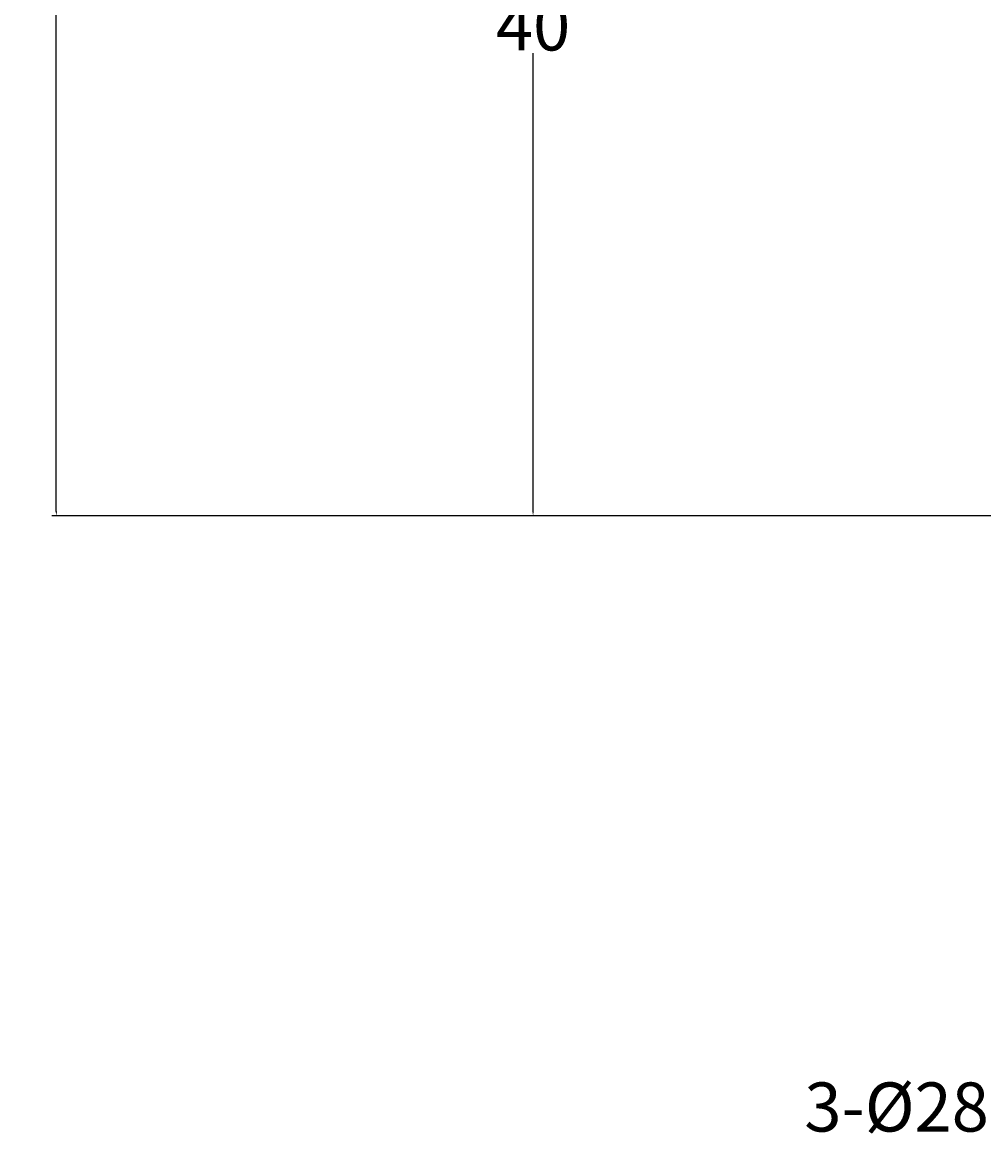
# Model space of a CAD drawing. Units: millimetres. Extents: x -60 to 113, y -37 to 126.
# Tile 1 of 17: x -60 to -21, y -18 to 27. Entities that reach past the tile are written whole.
import ezdxf

# ---------------------------------------------------------------- set-up
doc = ezdxf.new("R2010")
doc.units = ezdxf.units.MM
doc.header["$MEASUREMENT"] = 0
doc.layers.add('M-DIMS', color=2, linetype='Continuous', lineweight=25)
doc.styles.get("Standard").update_dxf_attribs({"font": 'arial.ttf'})
doc.dimstyles.get("Standard").update_dxf_attribs({"dimtxt": 0.18, "dimasz": 0.18, "dimexe": 0.18, "dimexo": 0.0625, "dimgap": 0.09, "dimtad": 0, "dimtih": 1, "dimtoh": 1, "dimdec": 4, "dimzin": 0, "dimdsep": 46, "dimtxsty": 'Standard', "dimcen": 0.09, "dimadec": 0, "dimazin": 0, "dimtfac": 1, "dimtdec": 4, "dimtofl": 0, "dimtmove": 0, "dimatfit": 3, "dimfxl": 1, "dimtolj": 1, "dimtzin": 0, "dimarcsym": 0})

# ---------------------------------------------------------------- blocks, each defined once
blk = doc.blocks.new('*D12')
at = {"layer": 'Defpoints', "color": 0, "transparency": 16777216}
for p in [(10.532, 88.533), (-58.719, 6.903), (11.329, 6.903)]:
    blk.add_point(p, dxfattribs=at)
at = {"layer": 'M-DIMS', "color": 0, "lineweight": -2, "transparency": 16777216}
for p, q in [((10.47, 88.533), (-58.899, 88.533)), ((-58.719, 88.353), (-58.719, 48.829)), ((-58.719, 7.083), (-58.719, 46.607)), ((11.267, 6.903), (-58.899, 6.903))]:
    blk.add_line(p, q, dxfattribs=at)
at = {"layer": 'M-DIMS', "color": 0, "transparency": 16777216}
for points in [[(-58.749, 88.353), (-58.689, 88.353), (-58.719, 88.533)], [(-58.749, 7.083), (-58.689, 7.083), (-58.719, 6.903)]]:
    blk.add_solid(points, dxfattribs=at)
at = {"layer": 'M-DIMS', "color": 0, "transparency": 16777216, "insert": (-58.719, 47.718), "char_height": 0.18, "attachment_point": 5}
blk.add_mtext('\\A1;{\\H11.11111x;82}', dxfattribs=at)
blk = doc.blocks.new('*D13')
at = {"layer": 'Defpoints', "color": 0, "transparency": 16777216}
for p in [(37.065, 46.813), (-39.303, 6.903), (7.267, 6.903)]:
    blk.add_point(p, dxfattribs=at)
at = {"layer": 'M-DIMS', "color": 0, "lineweight": -2, "transparency": 16777216}
for p, q in [((37.002, 46.813), (-39.483, 46.813)), ((-39.303, 46.633), (-39.303, 27.969)), ((-39.303, 7.083), (-39.303, 25.747)), ((7.204, 6.903), (-39.483, 6.903))]:
    blk.add_line(p, q, dxfattribs=at)
at = {"layer": 'M-DIMS', "color": 0, "transparency": 16777216}
for points in [[(-39.333, 46.633), (-39.273, 46.633), (-39.303, 46.813)], [(-39.333, 7.083), (-39.273, 7.083), (-39.303, 6.903)]]:
    blk.add_solid(points, dxfattribs=at)
at = {"layer": 'M-DIMS', "color": 0, "transparency": 16777216, "insert": (-39.303, 26.858), "char_height": 0.18, "attachment_point": 5}
blk.add_mtext('\\A1;{\\H11.11111x;40}', dxfattribs=at)
blk = doc.blocks.new('*D15')
at = {"layer": 'Defpoints', "color": 0, "transparency": 16777216}
for p in [(17.836, 16.083), (-3.303, -2.278)]:
    blk.add_point(p, dxfattribs=at)
at = {"layer": 'M-DIMS', "color": 0, "lineweight": -2, "transparency": 16777216}
for p, q in [((7.177, 6.903), (7.357, 6.903)), ((7.267, 6.813), (7.267, 6.993)), ((-20.464, -17.184), (-3.439, -2.396)), ((-20.644, -17.184), (-20.464, -17.184))]:
    blk.add_line(p, q, dxfattribs=at)
at = {"layer": 'M-DIMS', "color": 0, "transparency": 16777216}
blk.add_solid([(-3.459, -2.373), (-3.419, -2.419), (-3.303, -2.278)], dxfattribs=at)
at = {"layer": 'M-DIMS', "color": 0, "transparency": 16777216, "insert": (-24.497, -17.184), "char_height": 0.18, "attachment_point": 5}
blk.add_mtext('\\A1;{\\H11.11111x;3-%%C28}', dxfattribs=at)

msp = doc.modelspace()

# ---------------------------------------------------------------- dimensions: what is measured, and where the dimension line sits
at = {"layer": 'M-DIMS'}
for base, p1, p2, text, picture, middle in [((-58.71857, 6.9027), (10.53227, 88.53289), (11.32938, 6.9027), '{\\H11.11111x;82}', '*D12', (-58.71857, 47.71779)), ((-39.30316, 6.9027), (37.06463, 46.81263), (7.26659, 6.9027), '{\\H11.11111x;40}', '*D13', (-39.30316, 26.85766))]:
    dim = msp.add_linear_dim(base=base, p1=p1, p2=p2, angle=90, text=text, dimstyle='Standard', override={"dimclrd": 0, "dimclre": 0, "dimclrt": 0}, dxfattribs=at)
    dim.commit()
    dim.dimension.update_dxf_attribs({"geometry": picture, "text_midpoint": middle})
dim = msp.add_diameter_dim_2p(p1=(17.83613, 16.08337), p2=(-3.30296, -2.27798), text='{\\H11.11111x;3-%%C28}', dimstyle='Standard', override={"dimclrd": 0, "dimclre": 0, "dimclrt": 0}, dxfattribs=at)
dim.commit()
dim.dimension.update_dxf_attribs({"geometry": '*D15', "text_midpoint": (-24.49681, -17.18418), "dimtype": 163})

doc.saveas('drawing.dxf')
